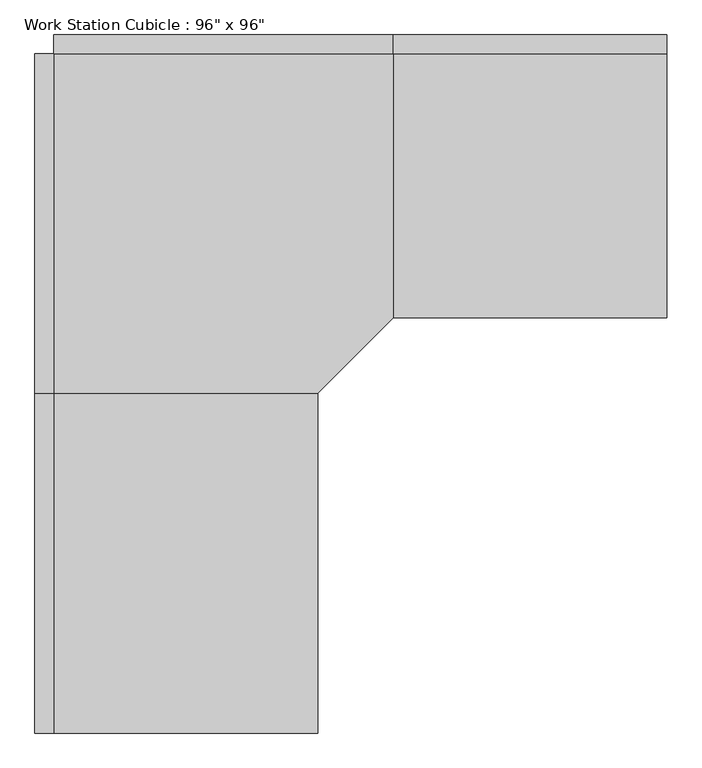
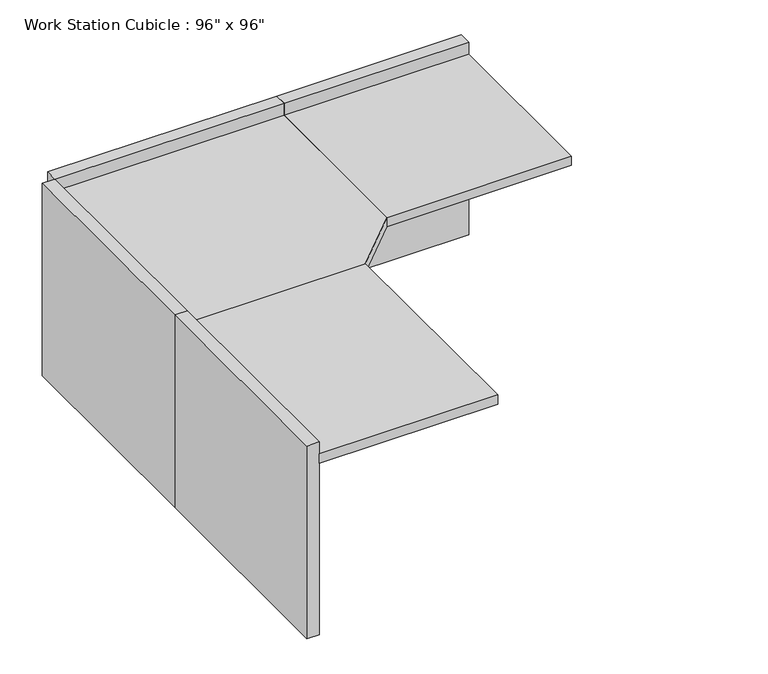
"""IFC4 building model written with IfcOpenShell, lengths in millimetres: furniture geometry."""

from ifc_helpers import new_model, si_unit, frame, origin, origin_with_axes, place, context, project, spatial, polyline, outline, extrude, source, transform, mapped, element, save


def furniture_005e41fd(model_context):
    return source(origin(), model_context, "Body", "SweptSolid", [
        extrude(outline(polyline([(-80.9317522, -545.8230076), (833.4682478, -545.8230076), (833.4682478, -1257.0230076), (630.2682478, -1460.2230076), (-80.9317522, -1460.2230076), (-80.9317522, -545.8230076)])), frame((0.0, 0.0, 723.9), z_axis=(0.0, 0.0, 1.0), x_axis=(1.0, 0.0, 0.0)), (0.0, 0.0, 1.0), 38.1),
        extrude(outline(polyline([(630.2682478, -2374.6230076), (-80.9317522, -2374.6230076), (-80.9317522, -1460.2230076), (630.2682478, -1460.2230076), (630.2682478, -2374.6230076)])), frame((0.0, 0.0, 723.9), z_axis=(0.0, 0.0, 1.0), x_axis=(1.0, 0.0, 0.0)), (0.0, 0.0, 1.0), 38.1),
        extrude(outline(polyline([(1570.0682478, -1257.0230076), (833.4682478, -1257.0230076), (833.4682478, -545.8230076), (1570.0682478, -545.8230076), (1570.0682478, -1257.0230076)])), frame((0.0, 0.0, 723.9), z_axis=(0.0, 0.0, 1.0), x_axis=(1.0, 0.0, 0.0)), (0.0, 0.0, 1.0), 38.1),
        extrude(outline(polyline([(1570.0682478, -545.8230076), (833.4682478, -545.8230076), (833.4682478, -495.0230076), (1570.0682478, -495.0230076), (1570.0682478, -545.8230076)])), origin_with_axes(), (0.0, 0.0, 1.0), 812.8),
        extrude(outline(polyline([(833.4682478, -545.8230076), (-80.9317522, -545.8230076), (-80.9317522, -495.0230076), (833.4682478, -495.0230076), (833.4682478, -545.8230076)])), origin_with_axes(), (0.0, 0.0, 1.0), 812.8),
        extrude(outline(polyline([(-80.9317522, -1460.2230076), (-131.7317522, -1460.2230076), (-131.7317522, -545.8230076), (-80.9317522, -545.8230076), (-80.9317522, -1460.2230076)])), origin_with_axes(), (0.0, 0.0, 1.0), 812.8),
        extrude(outline(polyline([(-80.9317522, -2374.6230076), (-131.7317522, -2374.6230076), (-131.7317522, -1460.2230076), (-80.9317522, -1460.2230076), (-80.9317522, -2374.6230076)])), origin_with_axes(), (0.0, 0.0, 1.0), 812.8),
    ])


if __name__ == "__main__":
    model = new_model("IFC4")
    model_context = context("Model", 3, world=origin())
    ifc_project = project(units=[si_unit("LENGTHUNIT", "METRE", prefix="MILLI")], contexts=[model_context])
    site = spatial("IfcSite", under=ifc_project)
    building = spatial("IfcBuilding", under=site)
    placement = place(None, origin())
    furniture_shape = furniture_005e41fd(model_context)
    element("IfcFurniture", 1, ObjectType="Work Station Cubicle : 96\" x 96\"", at=placement, inside=building, context=model_context, shape_type="MappedRepresentation", body=[
        mapped(furniture_shape, transform((0.0, 0.0, 0.0), x_axis=(1.0, 0.0, 0.0), y_axis=(0.0, 1.0, 0.0), z_axis=(0.0, 0.0, 1.0))),
    ])
    save(model, "model.ifc")

# Revit data of these elements
# Type "Work Station Cubicle : 96\" x 96\""
#   Assembly Code = "E2020"
#   Desktop Height = 2' - 6"
#   Desktop1 Width = 2' - 4"
#   Desktop2 Width = 2' - 4"
#   Panel Height = 2' - 8"
#   Panel1 Length = 3' - 0"
#   Panel2 Length = 2' - 5"
#   Cube Panel Material = Textile - Light Gray
#   Work Top Material = Laminate, Ivory, Matte
#   Default Elevation = 0
# Element 1 (IfcFurniture, "Work Station Cubicle : 96\" x 96\"")
#   Materials on its faces: "Textile - Light Gray", "Laminate, Ivory, Matte"
# Materials
#   "Textile - Light Gray": class "Fabric", colour RGB 204 204 204, transparency 0
#   "Laminate, Ivory, Matte": class "Plastic", colour RGB 247 247 239, transparency 0, Description = "Plastic Laminate - Ivory, Matte", Cost = 0
